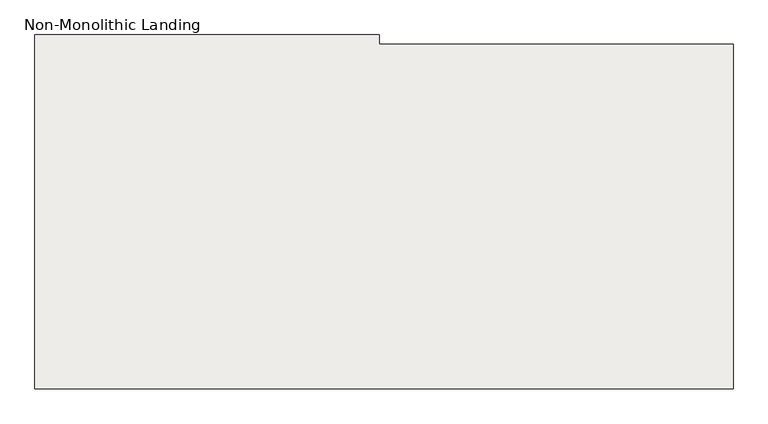
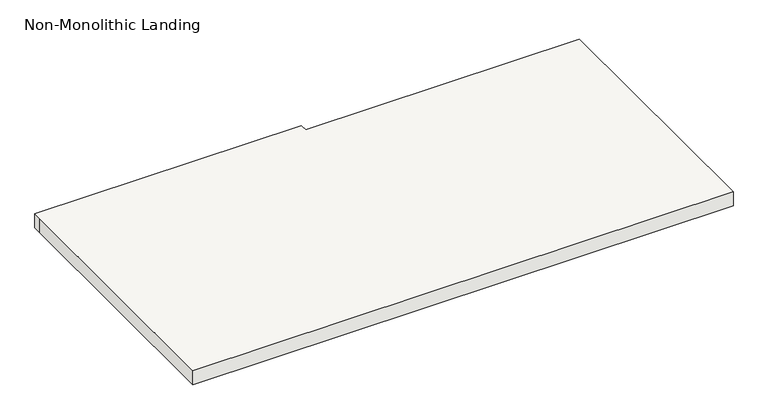
"""IFC4 building model written with IfcOpenShell, lengths in millimetres: slab geometry, Non-Monolithic Landing."""

from ifc_helpers import new_model, si_unit, origin, place, context, project, spatial, faceted_brep, source, transform, mapped, element, save


def non_monolithic_landing_419a9ad9(model_context):
    return source(origin(), model_context, "Body", "Brep", [
        faceted_brep([(15150.9506237, -3589.3064015, 5568.95), (15150.9506237, -3614.7064015, 5543.55), (14236.5506237, -3614.7064015, 5543.55), (14236.5506237, -3589.3064015, 5568.95), (14211.1506237, -3589.3064015, 5588.0), (14211.1506237, -3563.9064015, 5588.0), (13296.7506237, -3563.9064015, 5588.0), (13296.7506237, -3589.3064015, 5588.0), (13296.7506237, -4503.7064015, 5588.0), (15150.9506237, -4503.7064015, 5588.0), (15150.9506237, -3589.3064015, 5588.0), (14236.5506237, -3614.7064015, 5537.2), (15150.9506237, -3614.7064015, 5537.2), (15150.9506237, -4503.7064015, 5537.2), (13296.7506237, -4503.7064015, 5537.2), (13296.7506237, -3589.3064015, 5537.2), (13296.7506237, -3563.9064015, 5537.2), (14211.1506237, -3563.9064015, 5537.2), (14211.1506237, -3589.3064015, 5537.2), (14236.5506237, -3589.3064015, 5537.2)], [[[0, 1, 2, 3]], [[4, 5, 6, 7, 8, 9, 10]], [[11, 12, 13, 14, 15, 16, 17, 18, 19]], [[12, 11, 2, 1]], [[11, 19, 3, 2]], [[4, 10, 0, 3, 19, 18]], [[5, 4, 18, 17]], [[6, 5, 17, 16]], [[7, 6, 16, 15]], [[8, 7, 15, 14]], [[9, 8, 14, 13]], [[10, 9, 13, 12, 1, 0]]]),
    ])


if __name__ == "__main__":
    model = new_model("IFC4")
    model_context = context("Model", 3, world=origin())
    ifc_project = project(units=[si_unit("LENGTHUNIT", "METRE", prefix="MILLI")], contexts=[model_context])
    site = spatial("IfcSite", under=ifc_project)
    building = spatial("IfcBuilding", under=site)
    placement = place(None, origin())
    non_monolithic_landing_shape = non_monolithic_landing_419a9ad9(model_context)
    element("IfcSlab", 1, ObjectType="Non-Monolithic Landing", at=placement, inside=building, context=model_context, shape_type="MappedRepresentation", body=[
        mapped(non_monolithic_landing_shape, transform((0.0, 0.0, 0.0), x_axis=(1.0, 0.0, 0.0), y_axis=(0.0, 1.0, 0.0), z_axis=(0.0, 0.0, 1.0))),
    ])
    save(model, "model.ifc")
